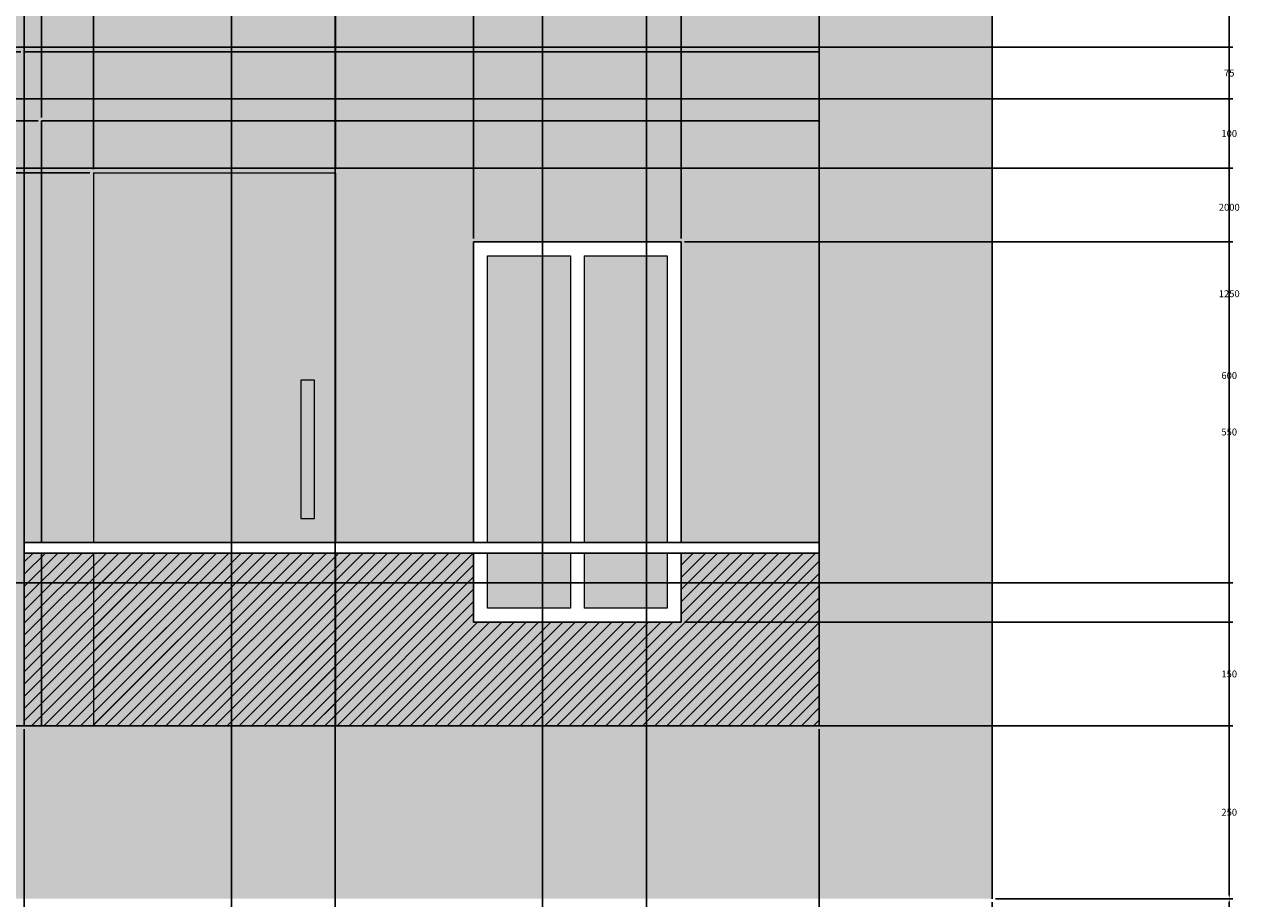
# Model space of a CAD drawing. Units: millimetres. Extents: x 2970 to 7764, y 2196 to 7505.
# Tile 11 of 13: x 6006 to 7764, y 5006 to 6270. Entities that reach past the tile are written whole.
import ezdxf

# ---------------------------------------------------------------- set-up
doc = ezdxf.new("R2010")
doc.units = ezdxf.units.MM
doc.header["$MEASUREMENT"] = 0
for name, color, linetype, lineweight in [('A-ANNO-DIMS', 2, 'Continuous', 18), ('A-DOOR', 3, 'Continuous', 18), ('A-ELEV', 7, 'Continuous', 25), ('A-ELEV-PATT', 8, 'Continuous', 13), ('A-GLAZ', 4, 'Continuous', 18)]:
    doc.layers.add(name, color=color, linetype=linetype, lineweight=lineweight)
doc.styles.get("Standard").update_dxf_attribs({"font": 'arial.ttf'})
doc.dimstyles.get("Standard").update_dxf_attribs({"dimtxt": 10, "dimasz": 5, "dimexe": 5, "dimexo": 5, "dimgap": 2, "dimtad": 0, "dimtih": 1, "dimtoh": 1, "dimdec": 0, "dimzin": 0, "dimdsep": 46, "dimtxsty": 'Standard', "dimcen": 2, "dimadec": 0, "dimazin": 0, "dimtfac": 1, "dimtdec": 0, "dimtofl": 0, "dimtmove": 0, "dimatfit": 3, "dimfxl": 1, "dimtolj": 1, "dimtzin": 0, "dimarcsym": 0})

# ---------------------------------------------------------------- blocks, each defined once
blk = doc.blocks.new('DOOR-HANDLE')
for p, q in [((20, 200), (0, 200)), ((0, 200), (0, 0)), ((20, 100), (20, 200)), ((20, 0), (20, 100)), ((0, 0), (20, 0))]:
    blk.add_line(p, q)
blk = doc.blocks.new('*D31')
at = {"layer": 'A-ANNO-DIMS', "color": 0, "lineweight": -2, "transparency": 16777216}
for p, q in [((7410.5, 5005.8), (7753.5, 5005.8)), ((7748.5, 5000.8), (7748.5, 4737.9)), ((7748.5, 4460.8), (7748.5, 4723.7)), ((7160.5, 4455.8), (7753.5, 4455.8))]:
    blk.add_line(p, q, dxfattribs=at)
at = {"layer": 'A-ANNO-DIMS', "color": 0, "transparency": 16777216}
for points in [[(7747.7, 5000.8), (7749.3, 5000.8), (7748.5, 5005.8)], [(7747.7, 4460.8), (7749.3, 4460.8), (7748.5, 4455.8)]]:
    blk.add_solid(points, dxfattribs=at)
at = {"layer": 'Defpoints', "color": 0, "transparency": 16777216}
for p in [(7405.5, 5005.8), (7748.5, 5005.8), (7155.5, 4455.8)]:
    blk.add_point(p, dxfattribs=at)
at = {"layer": 'A-ANNO-DIMS', "color": 0, "transparency": 16777216, "insert": (7748.5, 4730.8), "char_height": 10, "attachment_point": 5}
blk.add_mtext('\\A1;550', dxfattribs=at)
blk = doc.blocks.new('*D32')
at = {"layer": 'A-ANNO-DIMS', "color": 0, "lineweight": -2, "transparency": 16777216}
for p, q in [((6160.5, 7005.8), (7753.5, 7005.8)), ((7748.5, 7000.8), (7748.5, 6012.9)), ((7748.5, 5010.8), (7748.5, 5998.7)), ((7410.5, 5005.8), (7753.5, 5005.8))]:
    blk.add_line(p, q, dxfattribs=at)
at = {"layer": 'A-ANNO-DIMS', "color": 0, "transparency": 16777216}
for points in [[(7747.7, 7000.8), (7749.3, 7000.8), (7748.5, 7005.8)], [(7747.7, 5010.8), (7749.3, 5010.8), (7748.5, 5005.8)]]:
    blk.add_solid(points, dxfattribs=at)
at = {"layer": 'Defpoints', "color": 0, "transparency": 16777216}
for p in [(6155.5, 7005.8), (7748.5, 7005.8), (7405.5, 5005.8)]:
    blk.add_point(p, dxfattribs=at)
at = {"layer": 'A-ANNO-DIMS', "color": 0, "transparency": 16777216, "insert": (7748.5, 6005.8), "char_height": 10, "attachment_point": 5}
blk.add_mtext('\\A1;2000', dxfattribs=at)
blk = doc.blocks.new('*D38')
at = {"layer": 'A-ANNO-DIMS', "color": 0, "lineweight": -2, "transparency": 16777216}
for p, q in [((6755.3, 4010.8), (6755.3, 7503.8)), ((6760.3, 7498.8), (6808.1, 7498.8)), ((6900.5, 7498.8), (6852.7, 7498.8)), ((6905.5, 4210.8), (6905.5, 7503.8))]:
    blk.add_line(p, q, dxfattribs=at)
at = {"layer": 'A-ANNO-DIMS', "color": 0, "transparency": 16777216}
for points in [[(6760.3, 7499.6), (6760.3, 7498), (6755.3, 7498.8)], [(6900.5, 7499.6), (6900.5, 7498), (6905.5, 7498.8)]]:
    blk.add_solid(points, dxfattribs=at)
at = {"layer": 'Defpoints', "color": 0, "transparency": 16777216}
for p in [(6905.5, 7498.8), (6905.5, 4205.8), (6755.3, 4005.8)]:
    blk.add_point(p, dxfattribs=at)
at = {"layer": 'A-ANNO-DIMS', "color": 0, "transparency": 16777216, "insert": (6830.4, 7498.8), "char_height": 10, "attachment_point": 5}
blk.add_mtext('\\A1;150.23', dxfattribs=at)
blk = doc.blocks.new('*D39')
at = {"layer": 'A-ANNO-DIMS', "color": 0, "lineweight": -2, "transparency": 16777216}
for p, q in [((5955.3, 4010.8), (5955.3, 7503.8)), ((5960.3, 7498.8), (6117.2, 7498.8)), ((6300.3, 7498.8), (6143.3, 7498.8)), ((6305.3, 4010.8), (6305.3, 7503.8))]:
    blk.add_line(p, q, dxfattribs=at)
at = {"layer": 'A-ANNO-DIMS', "color": 0, "transparency": 16777216}
for points in [[(5960.3, 7499.6), (5960.3, 7498), (5955.3, 7498.8)], [(6300.3, 7499.6), (6300.3, 7498), (6305.3, 7498.8)]]:
    blk.add_solid(points, dxfattribs=at)
at = {"layer": 'Defpoints', "color": 0, "transparency": 16777216}
for p in [(6305.3, 7498.8), (5955.3, 4005.8), (6305.3, 4005.8)]:
    blk.add_point(p, dxfattribs=at)
at = {"layer": 'A-ANNO-DIMS', "color": 0, "transparency": 16777216, "insert": (6130.3, 7498.8), "char_height": 10, "attachment_point": 5}
blk.add_mtext('\\A1;350', dxfattribs=at)
blk = doc.blocks.new('*D40')
at = {"layer": 'A-ANNO-DIMS', "color": 0, "lineweight": -2, "transparency": 16777216}
for p, q in [((6305.3, 4010.8), (6305.3, 7503.8)), ((6310.3, 7498.8), (6367.7, 7498.8)), ((6450.3, 7498.8), (6392.8, 7498.8)), ((6455.3, 4010.8), (6455.3, 7503.8))]:
    blk.add_line(p, q, dxfattribs=at)
at = {"layer": 'A-ANNO-DIMS', "color": 0, "transparency": 16777216}
for points in [[(6310.3, 7499.6), (6310.3, 7498), (6305.3, 7498.8)], [(6450.3, 7499.6), (6450.3, 7498), (6455.3, 7498.8)]]:
    blk.add_solid(points, dxfattribs=at)
at = {"layer": 'Defpoints', "color": 0, "transparency": 16777216}
for p in [(6455.3, 7498.8), (6305.3, 4005.8), (6455.3, 4005.8)]:
    blk.add_point(p, dxfattribs=at)
at = {"layer": 'A-ANNO-DIMS', "color": 0, "transparency": 16777216, "insert": (6380.3, 7498.8), "char_height": 10, "attachment_point": 5}
blk.add_mtext('\\A1;150', dxfattribs=at)
blk = doc.blocks.new('*D41')
at = {"layer": 'A-ANNO-DIMS', "color": 0, "lineweight": -2, "transparency": 16777216}
for p, q in [((6455.3, 4010.8), (6455.3, 7503.8)), ((6460.3, 7498.8), (6592.2, 7498.8)), ((6750.3, 7498.8), (6618.3, 7498.8)), ((6755.3, 4010.8), (6755.3, 7503.8))]:
    blk.add_line(p, q, dxfattribs=at)
at = {"layer": 'A-ANNO-DIMS', "color": 0, "transparency": 16777216}
for points in [[(6460.3, 7499.6), (6460.3, 7498), (6455.3, 7498.8)], [(6750.3, 7499.6), (6750.3, 7498), (6755.3, 7498.8)]]:
    blk.add_solid(points, dxfattribs=at)
at = {"layer": 'Defpoints', "color": 0, "transparency": 16777216}
for p in [(6755.3, 7498.8), (6455.3, 4005.8), (6755.3, 4005.8)]:
    blk.add_point(p, dxfattribs=at)
at = {"layer": 'A-ANNO-DIMS', "color": 0, "transparency": 16777216, "insert": (6605.3, 7498.8), "char_height": 10, "attachment_point": 5}
blk.add_mtext('\\A1;300', dxfattribs=at)
blk = doc.blocks.new('*D59')
at = {"layer": 'A-ANNO-DIMS', "color": 0, "lineweight": -2, "transparency": 16777216}
for p, q in [((6005.5, 5250.8), (6005.5, 2197.8)), ((7155.5, 5250.8), (7155.5, 2197.8)), ((6010.5, 2202.8), (6564.1, 2202.8)), ((7150.5, 2202.8), (6596.9, 2202.8))]:
    blk.add_line(p, q, dxfattribs=at)
at = {"layer": 'A-ANNO-DIMS', "color": 0, "transparency": 16777216}
for points in [[(6010.5, 2203.6), (6010.5, 2202), (6005.5, 2202.8)], [(7150.5, 2203.6), (7150.5, 2202), (7155.5, 2202.8)]]:
    blk.add_solid(points, dxfattribs=at)
at = {"layer": 'Defpoints', "color": 0, "transparency": 16777216}
for p in [(6005.5, 5255.8), (7155.5, 5255.8), (7155.5, 2202.8)]:
    blk.add_point(p, dxfattribs=at)
at = {"layer": 'A-ANNO-DIMS', "color": 0, "transparency": 16777216, "insert": (6580.5, 2202.8), "char_height": 10, "attachment_point": 5}
blk.add_mtext('\\A1;1150', dxfattribs=at)
blk = doc.blocks.new('*D60')
at = {"layer": 'A-ANNO-DIMS', "color": 0, "lineweight": -2, "transparency": 16777216}
for p, q in [((7155.5, 5250.8), (7155.5, 2197.8)), ((7405.5, 5000.8), (7405.5, 2197.8)), ((7160.5, 2202.8), (7267.4, 2202.8)), ((7400.5, 2202.8), (7293.6, 2202.8))]:
    blk.add_line(p, q, dxfattribs=at)
at = {"layer": 'A-ANNO-DIMS', "color": 0, "transparency": 16777216}
for points in [[(7160.5, 2203.6), (7160.5, 2202), (7155.5, 2202.8)], [(7400.5, 2203.6), (7400.5, 2202), (7405.5, 2202.8)]]:
    blk.add_solid(points, dxfattribs=at)
at = {"layer": 'Defpoints', "color": 0, "transparency": 16777216}
for p in [(7155.5, 5255.8), (7405.5, 5005.8), (7405.5, 2202.8)]:
    blk.add_point(p, dxfattribs=at)
at = {"layer": 'A-ANNO-DIMS', "color": 0, "transparency": 16777216, "insert": (7280.5, 2202.8), "char_height": 10, "attachment_point": 5}
blk.add_mtext('\\A1;250', dxfattribs=at)
blk = doc.blocks.new('*D62')
at = {"layer": 'A-ANNO-DIMS', "color": 0, "lineweight": -2, "transparency": 16777216}
for p, q in [((5460.8, 6062.5), (7753.5, 6062.5)), ((7748.5, 6057.5), (7748.5, 5769.6)), ((7748.5, 5467.5), (7748.5, 5755.4)), ((5460.8, 5462.5), (7753.5, 5462.5))]:
    blk.add_line(p, q, dxfattribs=at)
at = {"layer": 'A-ANNO-DIMS', "color": 0, "transparency": 16777216}
for points in [[(7747.7, 6057.5), (7749.3, 6057.5), (7748.5, 6062.5)], [(7747.7, 5467.5), (7749.3, 5467.5), (7748.5, 5462.5)]]:
    blk.add_solid(points, dxfattribs=at)
at = {"layer": 'Defpoints', "color": 0, "transparency": 16777216}
for p in [(5455.8, 6062.5), (7748.5, 6062.5), (5455.8, 5462.5)]:
    blk.add_point(p, dxfattribs=at)
at = {"layer": 'A-ANNO-DIMS', "color": 0, "transparency": 16777216, "insert": (7748.5, 5762.5), "char_height": 10, "attachment_point": 5}
blk.add_mtext('\\A1;600', dxfattribs=at)
blk = doc.blocks.new('*D63')
at = {"layer": 'A-ANNO-DIMS', "color": 0, "lineweight": -2, "transparency": 16777216}
for p, q in [((5610.8, 6162.5), (7753.5, 6162.5)), ((7748.5, 6157.5), (7748.5, 6119.6)), ((7748.5, 6067.5), (7748.5, 6105.4)), ((5460.8, 6062.5), (7753.5, 6062.5))]:
    blk.add_line(p, q, dxfattribs=at)
at = {"layer": 'A-ANNO-DIMS', "color": 0, "transparency": 16777216}
for points in [[(7747.7, 6157.5), (7749.3, 6157.5), (7748.5, 6162.5)], [(7747.7, 6067.5), (7749.3, 6067.5), (7748.5, 6062.5)]]:
    blk.add_solid(points, dxfattribs=at)
at = {"layer": 'Defpoints', "color": 0, "transparency": 16777216}
for p in [(5605.8, 6162.5), (7748.5, 6162.5), (5455.8, 6062.5)]:
    blk.add_point(p, dxfattribs=at)
at = {"layer": 'A-ANNO-DIMS', "color": 0, "transparency": 16777216, "insert": (7748.5, 6112.5), "char_height": 10, "attachment_point": 5}
blk.add_mtext('\\A1;100', dxfattribs=at)
blk = doc.blocks.new('*D64')
at = {"layer": 'A-ANNO-DIMS', "color": 0, "lineweight": -2, "transparency": 16777216}
for p, q in [((5635.8, 6237.5), (7753.5, 6237.5)), ((7748.5, 6232.5), (7748.5, 6207.1)), ((7748.5, 6167.5), (7748.5, 6192.9)), ((5610.8, 6162.5), (7753.5, 6162.5))]:
    blk.add_line(p, q, dxfattribs=at)
at = {"layer": 'A-ANNO-DIMS', "color": 0, "transparency": 16777216}
for points in [[(7747.7, 6232.5), (7749.3, 6232.5), (7748.5, 6237.5)], [(7747.7, 6167.5), (7749.3, 6167.5), (7748.5, 6162.5)]]:
    blk.add_solid(points, dxfattribs=at)
at = {"layer": 'Defpoints', "color": 0, "transparency": 16777216}
for p in [(5630.8, 6237.5), (7748.5, 6237.5), (5605.8, 6162.5)]:
    blk.add_point(p, dxfattribs=at)
at = {"layer": 'A-ANNO-DIMS', "color": 0, "transparency": 16777216, "insert": (7748.5, 6200), "char_height": 10, "attachment_point": 5}
blk.add_mtext('\\A1;75', dxfattribs=at)
blk = doc.blocks.new('*D68')
at = {"layer": 'A-ANNO-DIMS', "color": 0, "lineweight": -2, "transparency": 16777216}
for p, q in [((7160.5, 5255.8), (7753.5, 5255.8)), ((7748.5, 5250.8), (7748.5, 5137.9)), ((7748.5, 5010.8), (7748.5, 5123.7)), ((7410.5, 5005.8), (7753.5, 5005.8))]:
    blk.add_line(p, q, dxfattribs=at)
at = {"layer": 'A-ANNO-DIMS', "color": 0, "transparency": 16777216}
for points in [[(7747.7, 5250.8), (7749.3, 5250.8), (7748.5, 5255.8)], [(7747.7, 5010.8), (7749.3, 5010.8), (7748.5, 5005.8)]]:
    blk.add_solid(points, dxfattribs=at)
at = {"layer": 'Defpoints', "color": 0, "transparency": 16777216}
for p in [(7155.5, 5255.8), (7748.5, 5255.8), (7405.5, 5005.8)]:
    blk.add_point(p, dxfattribs=at)
at = {"layer": 'A-ANNO-DIMS', "color": 0, "transparency": 16777216, "insert": (7748.5, 5130.8), "char_height": 10, "attachment_point": 5}
blk.add_mtext('\\A1;250', dxfattribs=at)
blk = doc.blocks.new('*D69')
at = {"layer": 'A-ANNO-DIMS', "color": 0, "lineweight": -2, "transparency": 16777216}
for p, q in [((7160.5, 6505.8), (7753.5, 6505.8)), ((7748.5, 6500.8), (7748.5, 5887.9)), ((7748.5, 5260.8), (7748.5, 5873.7)), ((7160.5, 5255.8), (7753.5, 5255.8))]:
    blk.add_line(p, q, dxfattribs=at)
at = {"layer": 'A-ANNO-DIMS', "color": 0, "transparency": 16777216}
for points in [[(7747.7, 6500.8), (7749.3, 6500.8), (7748.5, 6505.8)], [(7747.7, 5260.8), (7749.3, 5260.8), (7748.5, 5255.8)]]:
    blk.add_solid(points, dxfattribs=at)
at = {"layer": 'Defpoints', "color": 0, "transparency": 16777216}
for p in [(7155.5, 6505.8), (7748.5, 6505.8), (7155.5, 5255.8)]:
    blk.add_point(p, dxfattribs=at)
at = {"layer": 'A-ANNO-DIMS', "color": 0, "transparency": 16777216, "insert": (7748.5, 5880.8), "char_height": 10, "attachment_point": 5}
blk.add_mtext('\\A1;1250', dxfattribs=at)
blk = doc.blocks.new('*D71')
at = {"layer": 'A-ANNO-DIMS', "color": 0, "lineweight": -2, "transparency": 16777216}
for p, q in [((6030.5, 6135.8), (6030.5, 7503.8)), ((6035.5, 7498.8), (6058.8, 7498.8)), ((6100.5, 7498.8), (6077.2, 7498.8)), ((6105.5, 6060.8), (6105.5, 7503.8))]:
    blk.add_line(p, q, dxfattribs=at)
at = {"layer": 'A-ANNO-DIMS', "color": 0, "transparency": 16777216}
for points in [[(6035.5, 7499.6), (6035.5, 7498), (6030.5, 7498.8)], [(6100.5, 7499.6), (6100.5, 7498), (6105.5, 7498.8)]]:
    blk.add_solid(points, dxfattribs=at)
at = {"layer": 'Defpoints', "color": 0, "transparency": 16777216}
for p in [(6105.5, 7498.8), (6030.5, 6130.8), (6105.5, 6055.8)]:
    blk.add_point(p, dxfattribs=at)
at = {"layer": 'A-ANNO-DIMS', "color": 0, "transparency": 16777216, "insert": (6068, 7498.8), "char_height": 10, "attachment_point": 5}
blk.add_mtext('\\A1;75', dxfattribs=at)
blk = doc.blocks.new('*D72')
at = {"layer": 'A-ANNO-DIMS', "color": 0, "lineweight": -2, "transparency": 16777216}
for p, q in [((6105.5, 6060.8), (6105.5, 7503.8)), ((6110.5, 7498.8), (6267.5, 7498.8)), ((6450.5, 7498.8), (6293.5, 7498.8)), ((6455.5, 6060.8), (6455.5, 7503.8))]:
    blk.add_line(p, q, dxfattribs=at)
at = {"layer": 'A-ANNO-DIMS', "color": 0, "transparency": 16777216}
for points in [[(6110.5, 7499.6), (6110.5, 7498), (6105.5, 7498.8)], [(6450.5, 7499.6), (6450.5, 7498), (6455.5, 7498.8)]]:
    blk.add_solid(points, dxfattribs=at)
at = {"layer": 'Defpoints', "color": 0, "transparency": 16777216}
for p in [(6455.5, 7498.8), (6105.5, 6055.8), (6455.5, 6055.8)]:
    blk.add_point(p, dxfattribs=at)
at = {"layer": 'A-ANNO-DIMS', "color": 0, "transparency": 16777216, "insert": (6280.5, 7498.8), "char_height": 10, "attachment_point": 5}
blk.add_mtext('\\A1;350', dxfattribs=at)
blk = doc.blocks.new('*D73')
at = {"layer": 'A-ANNO-DIMS', "color": 0, "lineweight": -2, "transparency": 16777216}
for p, q in [((6455.5, 6060.8), (6455.5, 7503.8)), ((6460.5, 7498.8), (6542.4, 7498.8)), ((6650.5, 7498.8), (6568.6, 7498.8)), ((6655.5, 5960.8), (6655.5, 7503.8))]:
    blk.add_line(p, q, dxfattribs=at)
at = {"layer": 'A-ANNO-DIMS', "color": 0, "transparency": 16777216}
for points in [[(6460.5, 7499.6), (6460.5, 7498), (6455.5, 7498.8)], [(6650.5, 7499.6), (6650.5, 7498), (6655.5, 7498.8)]]:
    blk.add_solid(points, dxfattribs=at)
at = {"layer": 'Defpoints', "color": 0, "transparency": 16777216}
for p in [(6655.5, 7498.8), (6455.5, 6055.8), (6655.5, 5955.8)]:
    blk.add_point(p, dxfattribs=at)
at = {"layer": 'A-ANNO-DIMS', "color": 0, "transparency": 16777216, "insert": (6555.5, 7498.8), "char_height": 10, "attachment_point": 5}
blk.add_mtext('\\A1;200', dxfattribs=at)
blk = doc.blocks.new('*D74')
at = {"layer": 'A-ANNO-DIMS', "color": 0, "lineweight": -2, "transparency": 16777216}
for p, q in [((6655.5, 5960.8), (6655.5, 7503.8)), ((6660.5, 7498.8), (6792.5, 7498.8)), ((6950.5, 7498.8), (6818.5, 7498.8)), ((6955.5, 5960.8), (6955.5, 7503.8))]:
    blk.add_line(p, q, dxfattribs=at)
at = {"layer": 'A-ANNO-DIMS', "color": 0, "transparency": 16777216}
for points in [[(6660.5, 7499.6), (6660.5, 7498), (6655.5, 7498.8)], [(6950.5, 7499.6), (6950.5, 7498), (6955.5, 7498.8)]]:
    blk.add_solid(points, dxfattribs=at)
at = {"layer": 'Defpoints', "color": 0, "transparency": 16777216}
for p in [(6955.5, 7498.8), (6655.5, 5955.8), (6955.5, 5955.8)]:
    blk.add_point(p, dxfattribs=at)
at = {"layer": 'A-ANNO-DIMS', "color": 0, "transparency": 16777216, "insert": (6805.5, 7498.8), "char_height": 10, "attachment_point": 5}
blk.add_mtext('\\A1;300', dxfattribs=at)
blk = doc.blocks.new('*D75')
at = {"layer": 'A-ANNO-DIMS', "color": 0, "lineweight": -2, "transparency": 16777216}
for p, q in [((6955.5, 5960.8), (6955.5, 7503.8)), ((6960.5, 7498.8), (7042.4, 7498.8)), ((7150.5, 7498.8), (7068.6, 7498.8)), ((7155.5, 5260.8), (7155.5, 7503.8))]:
    blk.add_line(p, q, dxfattribs=at)
at = {"layer": 'A-ANNO-DIMS', "color": 0, "transparency": 16777216}
for points in [[(6960.5, 7499.6), (6960.5, 7498), (6955.5, 7498.8)], [(7150.5, 7499.6), (7150.5, 7498), (7155.5, 7498.8)]]:
    blk.add_solid(points, dxfattribs=at)
at = {"layer": 'Defpoints', "color": 0, "transparency": 16777216}
for p in [(7155.5, 7498.8), (6955.5, 5955.8), (7155.5, 5255.8)]:
    blk.add_point(p, dxfattribs=at)
at = {"layer": 'A-ANNO-DIMS', "color": 0, "transparency": 16777216, "insert": (7055.5, 7498.8), "char_height": 10, "attachment_point": 5}
blk.add_mtext('\\A1;200', dxfattribs=at)
blk = doc.blocks.new('*D76')
at = {"layer": 'A-ANNO-DIMS', "color": 0, "lineweight": -2, "transparency": 16777216}
for p, q in [((6100.5, 6055.8), (2982.5, 6055.8)), ((2987.5, 6050.8), (2987.5, 5662.9)), ((2987.5, 5260.8), (2987.5, 5648.7)), ((6100.5, 5255.8), (2982.5, 5255.8))]:
    blk.add_line(p, q, dxfattribs=at)
at = {"layer": 'A-ANNO-DIMS', "color": 0, "transparency": 16777216}
for points in [[(2986.7, 6050.8), (2988.3, 6050.8), (2987.5, 6055.8)], [(2986.7, 5260.8), (2988.3, 5260.8), (2987.5, 5255.8)]]:
    blk.add_solid(points, dxfattribs=at)
at = {"layer": 'Defpoints', "color": 0, "transparency": 16777216}
for p in [(2987.5, 6055.8), (6105.5, 6055.8), (6105.5, 5255.8)]:
    blk.add_point(p, dxfattribs=at)
at = {"layer": 'A-ANNO-DIMS', "color": 0, "transparency": 16777216, "insert": (2987.5, 5655.8), "char_height": 10, "attachment_point": 5}
blk.add_mtext('\\A1;800', dxfattribs=at)
blk = doc.blocks.new('*D77')
at = {"layer": 'A-ANNO-DIMS', "color": 0, "lineweight": -2, "transparency": 16777216}
for p, q in [((6960.5, 5405.8), (7753.5, 5405.8)), ((7748.5, 5400.8), (7748.5, 5337.9)), ((7748.5, 5260.8), (7748.5, 5323.7)), ((6010.5, 5255.8), (7753.5, 5255.8))]:
    blk.add_line(p, q, dxfattribs=at)
at = {"layer": 'A-ANNO-DIMS', "color": 0, "transparency": 16777216}
for points in [[(7747.7, 5400.8), (7749.3, 5400.8), (7748.5, 5405.8)], [(7747.7, 5260.8), (7749.3, 5260.8), (7748.5, 5255.8)]]:
    blk.add_solid(points, dxfattribs=at)
at = {"layer": 'Defpoints', "color": 0, "transparency": 16777216}
for p in [(6955.5, 5405.8), (7748.5, 5405.8), (6005.5, 5255.8)]:
    blk.add_point(p, dxfattribs=at)
at = {"layer": 'A-ANNO-DIMS', "color": 0, "transparency": 16777216, "insert": (7748.5, 5330.8), "char_height": 10, "attachment_point": 5}
blk.add_mtext('\\A1;150', dxfattribs=at)
blk = doc.blocks.new('*D78')
at = {"layer": 'A-ANNO-DIMS', "color": 0, "lineweight": -2, "transparency": 16777216}
for p, q in [((6960.5, 5955.8), (7753.5, 5955.8)), ((7748.5, 5950.8), (7748.5, 5687.9)), ((7748.5, 5410.8), (7748.5, 5673.7)), ((6960.5, 5405.8), (7753.5, 5405.8))]:
    blk.add_line(p, q, dxfattribs=at)
at = {"layer": 'A-ANNO-DIMS', "color": 0, "transparency": 16777216}
for points in [[(7747.7, 5950.8), (7749.3, 5950.8), (7748.5, 5955.8)], [(7747.7, 5410.8), (7749.3, 5410.8), (7748.5, 5405.8)]]:
    blk.add_solid(points, dxfattribs=at)
at = {"layer": 'Defpoints', "color": 0, "transparency": 16777216}
for p in [(6955.5, 5955.8), (7748.5, 5955.8), (6955.5, 5405.8)]:
    blk.add_point(p, dxfattribs=at)
at = {"layer": 'A-ANNO-DIMS', "color": 0, "transparency": 16777216, "insert": (7748.5, 5680.8), "char_height": 10, "attachment_point": 5}
blk.add_mtext('\\A1;550', dxfattribs=at)
blk = doc.blocks.new('*D81')
at = {"layer": 'A-ANNO-DIMS', "color": 0, "lineweight": -2, "transparency": 16777216}
for p, q in [((6000.5, 6230.8), (2982.5, 6230.8)), ((2987.5, 6225.8), (2987.5, 6187.9)), ((2987.5, 6135.8), (2987.5, 6173.7)), ((6025.5, 6130.8), (2982.5, 6130.8))]:
    blk.add_line(p, q, dxfattribs=at)
at = {"layer": 'A-ANNO-DIMS', "color": 0, "transparency": 16777216}
for points in [[(2986.7, 6225.8), (2988.3, 6225.8), (2987.5, 6230.8)], [(2986.7, 6135.8), (2988.3, 6135.8), (2987.5, 6130.8)]]:
    blk.add_solid(points, dxfattribs=at)
at = {"layer": 'Defpoints', "color": 0, "transparency": 16777216}
for p in [(2987.5, 6230.8), (6005.5, 6230.8), (6030.5, 6130.8)]:
    blk.add_point(p, dxfattribs=at)
at = {"layer": 'A-ANNO-DIMS', "color": 0, "transparency": 16777216, "insert": (2987.5, 6180.8), "char_height": 10, "attachment_point": 5}
blk.add_mtext('\\A1;100', dxfattribs=at)

msp = doc.modelspace()

# ---------------------------------------------------------------- hatches: boundary and pattern name
at = {"layer": 'A-ELEV-PATT'}
h = msp.add_hatch(color=256, dxfattribs=at)
h.dxf.hatch_style = 1
h.paths.add_polyline_path([(6405.5, 7255.789), (4305.5, 7255.789), (4305.5, 6505.789), (3730.5, 6505.789), (3730.5, 4205.789), (3730.5, 2945.789), (3730.5, 2895.789), (3830.5, 2895.789), (3830.5, 4205.789), (3830.5, 6405.789), (4405.5, 6405.789), (4405.5, 4205.789), (6905.5, 4205.789), (6905.5, 2945.789), (6905.5, 2845.789), (7155.5, 2845.789), (7155.5, 2945.789), (7155.5, 4205.789), (7155.5, 4455.789), (4555.5, 4455.789), (4555.5, 6505.789), (4555.5, 7005.789), (6155.5, 7005.789), (6155.5, 6755.789), (6405.5, 6755.789)])
h.paths.add_polyline_path([(7405.5, 6755.789), (6155.5, 6755.789), (5755.5, 6755.789), (5755.5, 5005.789), (7405.5, 5005.789)])
h.paths.add_polyline_path([(7155.5, 6505.789), (7155.5, 5255.789), (6005.5, 5255.789), (6005.5, 6505.789)], flags=16)
h.paths.add_polyline_path([(6105.5, 5520.789), (6105.5, 6055.789), (6455.5, 6055.789), (6455.5, 5520.789), (6655.5, 5520.789), (6655.5, 5605.789), (6655.5, 5955.789), (6955.5, 5955.789), (6955.5, 5605.789), (6955.5, 5520.789)], flags=0)
h.paths.add_polyline_path([(6425.5, 5755.789), (6425.5, 5655.789), (6425.5, 5555.789), (6405.5, 5555.789), (6405.5, 5755.789)], flags=0)
h.paths.add_polyline_path([(6955.5, 5505.789), (6955.5, 5405.789), (6655.5, 5405.789), (6655.5, 5505.789)], flags=0)
h = msp.add_hatch(color=256, dxfattribs=at)
h.set_gradient(color1=(19, 76, 0), color2=(0, 127, 31), name='INVCURVED')
h.paths.add_polyline_path([(6005.5, 6505.789), (6005.5, 6230.789), (7155.5, 6230.789), (7155.5, 6505.789)])
h = msp.add_hatch(color=256, dxfattribs=at)
h.set_gradient(color1=(147, 149, 152), color2=(31, 31, 31), name='CURVED')
h.paths.add_polyline_path([(6005.5, 6230.789), (6005.5, 5520.789), (6030.5, 5520.789), (6030.5, 6130.789), (7155.5, 6130.789), (7155.5, 6230.789)])
h.paths.add_polyline_path([(6030.5, 5255.789), (6030.5, 5505.789), (6005.5, 5505.789), (6005.5, 5255.789)])
h = msp.add_hatch(color=256, dxfattribs=at)
h.set_gradient(color1=(99, 100, 102), color2=(147, 149, 152), name='INVCURVED')
h.paths.add_polyline_path([(6455.5, 5520.789), (6655.5, 5520.789), (6655.5, 5605.789), (6655.5, 5955.789), (6955.5, 5955.789), (6955.5, 5605.789), (6955.5, 5520.789), (7155.5, 5520.789), (7155.5, 6130.789), (6030.5, 6130.789), (6030.5, 5520.789), (6105.5, 5520.789), (6105.5, 6055.789), (6455.5, 6055.789)])
h.paths.add_polyline_path([(6655.5, 5405.789), (6655.5, 5505.789), (6455.5, 5505.789), (6455.5, 5255.789), (7155.5, 5255.789), (7155.5, 5505.789), (6955.5, 5505.789), (6955.5, 5405.789)])
h.paths.add_polyline_path([(6105.5, 5505.789), (6030.5, 5505.789), (6030.5, 5255.789), (6105.5, 5255.789)])
h = msp.add_hatch(color=256, dxfattribs=at)
h.set_gradient(color1=(153, 76, 0), color2=(204, 102, 0))
h.paths.add_polyline_path([(6455.5, 6055.789), (6105.5, 6055.789), (6105.5, 5520.789), (6455.5, 5520.789)])
h.paths.add_polyline_path([(6405.5, 5755.789), (6425.5, 5755.789), (6425.5, 5655.789), (6425.5, 5555.789), (6405.5, 5555.789)], flags=16)
h.paths.add_polyline_path([(6455.5, 5255.789), (6455.5, 5505.789), (6105.5, 5505.789), (6105.5, 5255.789)])
h = msp.add_hatch(color=256, dxfattribs=at)
h.set_gradient(color1=(122, 175, 223), color2=(173, 221, 247), name='SPHERICAL')
h.paths.add_polyline_path([(6675.5, 5605.789), (6675.5, 5520.789), (6795.5, 5520.789), (6795.5, 5605.789), (6795.5, 5935.789), (6675.5, 5935.789)])
h.paths.add_polyline_path([(6815.5, 5605.789), (6815.5, 5520.789), (6935.5, 5520.789), (6935.5, 5605.789), (6935.5, 5935.789), (6815.5, 5935.789)])
h.paths.add_polyline_path([(6935.5, 5425.789), (6935.5, 5505.789), (6815.5, 5505.789), (6815.5, 5425.789)])
h.paths.add_polyline_path([(6675.5, 5505.789), (6675.5, 5425.789), (6795.5, 5425.789), (6795.5, 5505.789)])
h = msp.add_hatch(color=256, dxfattribs=at)
h.set_gradient(color1=(248, 215, 49), color2=(247, 242, 129), name='SPHERICAL')
h.paths.add_polyline_path([(6425.5, 5755.789), (6405.5, 5755.789), (6405.5, 5555.789), (6425.5, 5555.789), (6425.5, 5655.789)])
h = msp.add_hatch(dxfattribs=at)
h.set_pattern_fill('ANSI31', color=256, scale=100, style=0)
h.paths.add_polyline_path([(7155.5, 5505.789), (6955.5, 5505.789), (6955.5, 5405.789), (6655.5, 5405.789), (6655.5, 5505.789), (6455.5, 5505.789), (6455.5, 5255.789), (7155.5, 5255.789)])
h.paths.add_polyline_path([(6455.5, 5505.789), (6105.5, 5505.789), (6105.5, 5255.789), (6455.5, 5255.789)])
h.paths.add_polyline_path([(6105.5, 5505.789), (6030.5, 5505.789), (6030.5, 5255.789), (6105.5, 5255.789)])
h.paths.add_polyline_path([(6030.5, 5505.789), (6005.5, 5505.789), (6005.5, 5255.789), (6030.5, 5255.789)])
h = msp.add_hatch(dxfattribs=at)
h.set_pattern_fill('ANSI31', color=256, scale=100, style=0)
h.paths.add_polyline_path([(6455.5, 5505.789), (6105.5, 5505.789), (6105.5, 5255.789), (6455.5, 5255.789)])

# ---------------------------------------------------------------- linework, layer by layer
at = {"layer": 'A-DOOR'}
for p, q in [((6105.5, 6055.789), (6105.5, 5520.789)), ((6105.5, 6055.789), (6455.5, 6055.789)), ((6455.5, 6055.789), (6455.5, 5520.789)), ((6105.5, 5505.789), (6105.5, 5255.789)), ((6455.5, 5505.789), (6455.5, 5255.789))]:
    msp.add_line(p, q, dxfattribs=at)
at = {"layer": 'A-ELEV'}
for p, q in [((7405.5, 6755.789), (7405.5, 5005.789)), ((6005.5, 5255.789), (6005.5, 6505.789)), ((7155.5, 6505.789), (7155.5, 5255.789)), ((6005.5, 6230.789), (7155.5, 6230.789)), ((6030.5, 6130.789), (7155.5, 6130.789)), ((6030.5, 5520.789), (6030.5, 6130.789)), ((7155.5, 5520.789), (6005.5, 5520.789)), ((7155.5, 5505.789), (6005.5, 5505.789)), ((6030.5, 5255.789), (6030.5, 5505.789)), ((7155.5, 5255.789), (6005.5, 5255.789))]:
    msp.add_line(p, q, dxfattribs=at)
for points in [[(6655.5, 5605.789), (6655.5, 5955.789), (6955.5, 5955.789), (6955.5, 5605.789)], [(6655.5, 5520.789), (6655.5, 5605.789)], [(6955.5, 5605.789), (6955.5, 5520.789)], [(6955.5, 5505.789), (6955.5, 5405.789), (6655.5, 5405.789), (6655.5, 5505.789)]]:
    msp.add_lwpolyline(points, dxfattribs=at)
at = {"layer": 'A-GLAZ'}
for p, q in [((6795.5, 5935.789), (6795.5, 5605.789)), ((6815.5, 5935.789), (6815.5, 5605.789)), ((6795.5, 5605.789), (6795.5, 5520.789)), ((6815.5, 5605.789), (6815.5, 5520.789)), ((6795.5, 5505.789), (6795.5, 5425.789)), ((6815.5, 5505.789), (6815.5, 5425.789))]:
    msp.add_line(p, q, dxfattribs=at)
for points in [[(6675.5, 5605.789), (6675.5, 5935.789), (6795.5, 5935.789)], [(6815.5, 5935.789), (6935.5, 5935.789), (6935.5, 5605.789)], [(6675.5, 5520.789), (6675.5, 5605.789)], [(6935.5, 5605.789), (6935.5, 5520.789)], [(6795.5, 5425.789), (6675.5, 5425.789), (6675.5, 5505.789)], [(6935.5, 5505.789), (6935.5, 5425.789), (6815.5, 5425.789)]]:
    msp.add_lwpolyline(points, dxfattribs=at)

# ---------------------------------------------------------------- block references
at = {"layer": 'A-DOOR'}
msp.add_blockref('DOOR-HANDLE', (6405.5, 5555.789), dxfattribs=at)

# ---------------------------------------------------------------- dimensions: what is measured, and where the dimension line sits
at = {"layer": 'A-ANNO-DIMS'}
for base, p1, p2, override, picture, middle in [((6305.271, 7498.789), (5955.271, 4005.789), (6305.271, 4005.789), {"dimdec": 0, "dimlfac": 1, "dimrnd": 0, "dimzin": 0, "dimdsep": 46, "dimlunit": 2}, '*D39', (6130.271, 7498.789)), ((6105.5, 7498.789), (6030.5, 6130.789), (6105.5, 6055.789), {"dimdec": 0, "dimlfac": 1, "dimrnd": 0, "dimzin": 0, "dimdsep": 46, "dimlunit": 2}, '*D71', (6068, 7498.789)), ((6455.5, 7498.789), (6105.5, 6055.789), (6455.5, 6055.789), {"dimdec": 0, "dimlfac": 1, "dimrnd": 0, "dimzin": 0, "dimdsep": 46, "dimlunit": 2}, '*D72', (6280.5, 7498.789)), ((6455.271, 7498.789), (6305.271, 4005.789), (6455.271, 4005.789), {"dimdec": 0, "dimlfac": 1, "dimrnd": 0, "dimzin": 0, "dimdsep": 46, "dimlunit": 2}, '*D40', (6380.271, 7498.789)), ((6755.271, 7498.789), (6455.271, 4005.789), (6755.271, 4005.789), {"dimdec": 0, "dimlfac": 1, "dimrnd": 0, "dimzin": 0, "dimdsep": 46, "dimlunit": 2}, '*D41', (6605.271, 7498.789)), ((6655.5, 7498.789), (6455.5, 6055.789), (6655.5, 5955.789), {"dimdec": 0, "dimlfac": 1, "dimrnd": 0, "dimzin": 0, "dimdsep": 46, "dimlunit": 2}, '*D73', (6555.5, 7498.789)), ((6955.5, 7498.789), (6655.5, 5955.789), (6955.5, 5955.789), {"dimdec": 0, "dimlfac": 1, "dimrnd": 0, "dimzin": 0, "dimdsep": 46, "dimlunit": 2}, '*D74', (6805.5, 7498.789)), ((6905.5, 7498.789), (6755.271, 4005.789), (6905.5, 4205.789), {"dimdec": 2, "dimlfac": 1, "dimrnd": 0, "dimzin": 0, "dimdsep": 46, "dimlunit": 2}, '*D38', (6830.386, 7498.789)), ((7155.5, 7498.789), (6955.5, 5955.789), (7155.5, 5255.789), {"dimdec": 0, "dimlfac": 1, "dimrnd": 0, "dimzin": 0, "dimdsep": 46, "dimlunit": 2}, '*D75', (7055.5, 7498.789)), ((7155.5, 2202.789), (6005.5, 5255.789), (7155.5, 5255.789), {"dimdec": 0, "dimlfac": 1, "dimrnd": 0, "dimzin": 0, "dimdsep": 46, "dimlunit": 2}, '*D59', (6580.5, 2202.789)), ((7405.5, 2202.789), (7155.5, 5255.789), (7405.5, 5005.789), {"dimdec": 0, "dimlfac": 1, "dimrnd": 0, "dimzin": 0, "dimdsep": 46, "dimlunit": 2}, '*D60', (7280.5, 2202.789))]:
    dim = msp.add_linear_dim(base=base, p1=p1, p2=p2, dimstyle='Standard', override=override, dxfattribs=at)
    dim.commit()
    dim.dimension.update_dxf_attribs({"geometry": picture, "text_midpoint": middle})
for base, p1, p2, picture, middle in [((7748.5, 7005.789), (7405.5, 5005.789), (6155.5, 7005.789), '*D32', (7748.5, 6005.789)), ((7748.5, 6505.789), (7155.5, 5255.789), (7155.5, 6505.789), '*D69', (7748.5, 5880.789)), ((2987.5, 6230.789), (6030.5, 6130.789), (6005.5, 6230.789), '*D81', (2987.5, 6180.789)), ((7748.5, 6237.49), (5605.81, 6162.49), (5630.81, 6237.49), '*D64', (7748.5, 6199.99)), ((7748.5, 6162.49), (5455.81, 6062.49), (5605.81, 6162.49), '*D63', (7748.5, 6112.49)), ((2987.5, 6055.789), (6105.5, 5255.789), (6105.5, 6055.789), '*D76', (2987.5, 5655.789)), ((7748.5, 6062.49), (5455.81, 5462.49), (5455.81, 6062.49), '*D62', (7748.5, 5762.49)), ((7748.5, 5955.789), (6955.5, 5405.789), (6955.5, 5955.789), '*D78', (7748.5, 5680.789)), ((7748.5, 5405.789), (6005.5, 5255.789), (6955.5, 5405.789), '*D77', (7748.5, 5330.789)), ((7748.5, 5255.789), (7405.5, 5005.789), (7155.5, 5255.789), '*D68', (7748.5, 5130.789)), ((7748.5, 5005.789), (7155.5, 4455.789), (7405.5, 5005.789), '*D31', (7748.5, 4730.789))]:
    dim = msp.add_linear_dim(base=base, p1=p1, p2=p2, angle=90, dimstyle='Standard', override={"dimdec": 0, "dimlfac": 1, "dimrnd": 0, "dimzin": 0, "dimdsep": 46, "dimlunit": 2}, dxfattribs=at)
    dim.commit()
    dim.dimension.update_dxf_attribs({"geometry": picture, "text_midpoint": middle})

doc.saveas('drawing.dxf')
